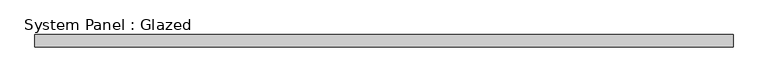
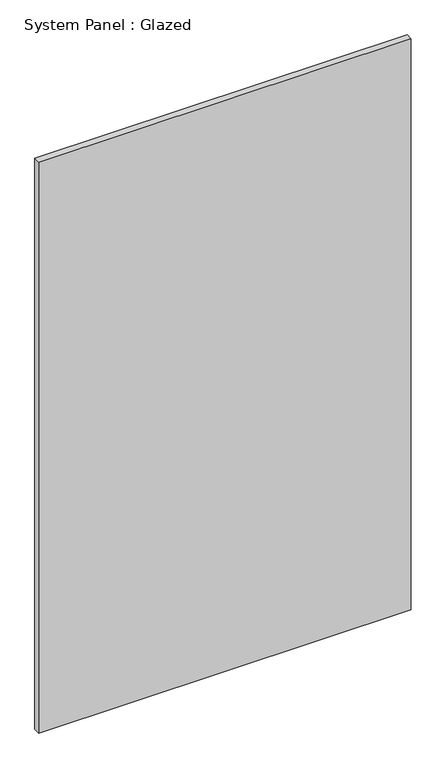
"""IFC4 building model written with IfcOpenShell, lengths in millimetres: plate geometry, System Panel : Glazed."""

from ifc_helpers import new_model, si_unit, origin, origin_with_axes, place, context, project, spatial, polyline, outline, extrude, source, transform, mapped, element, save


def system_panel_glazed_8fc861e4(model_context):
    return source(origin(), model_context, "Body", "SweptSolid", [
        extrude(outline(polyline([(723.4907433, -44.45), (-723.4907433, -44.45), (-723.4907433, -19.05), (723.4907433, -19.05), (723.4907433, -44.45)])), origin_with_axes(), (0.0, 0.0, 1.0), 2343.15),
    ])


if __name__ == "__main__":
    model = new_model("IFC4")
    model_context = context("Model", 3, world=origin())
    ifc_project = project(units=[si_unit("LENGTHUNIT", "METRE", prefix="MILLI")], contexts=[model_context])
    site = spatial("IfcSite", under=ifc_project)
    building = spatial("IfcBuilding", under=site)
    placement = place(None, origin())
    system_panel_glazed_shape = system_panel_glazed_8fc861e4(model_context)
    element("IfcPlate", 1, ObjectType="System Panel : Glazed", at=placement, inside=building, context=model_context, shape_type="MappedRepresentation", body=[
        mapped(system_panel_glazed_shape, transform((0.0, 0.0, 0.0), x_axis=(1.0, 0.0, 0.0), y_axis=(0.0, 1.0, 0.0), z_axis=(0.0, 0.0, 1.0))),
    ])
    save(model, "model.ifc")

# Revit data of these elements
# Type "System Panel : Glazed"
#   Construction Type Id = "GSP4R"
#   Analytic Construction = "1/8 in Pilkington single glazing"
#   Visual Light Transmittance = 0.9
#   Solar Heat Gain Coefficient = 0.86
#   Heat Transfer Coefficient (U) = 1.18115 BTU/(h·ft²·°F)
# Element 1 (IfcPlate, "System Panel : Glazed")
#   Materials on its faces: "Glass"
# Materials
#   "Glass": class "Glass", colour RGB 0 128 192, transparency 0.75, Description = "Soda Lime Glass", Cost = 0
